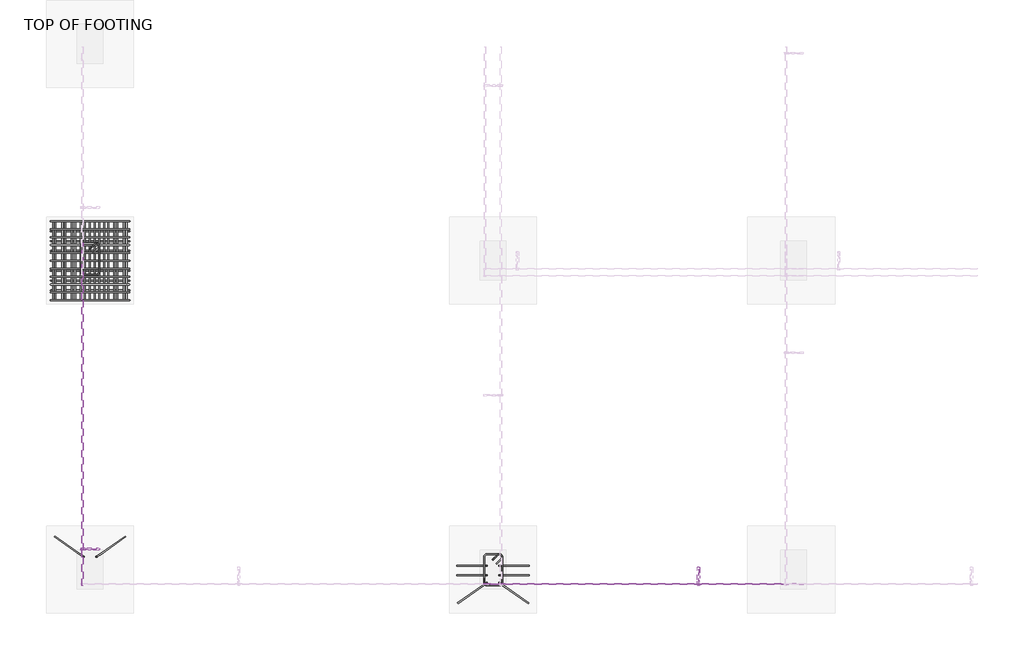
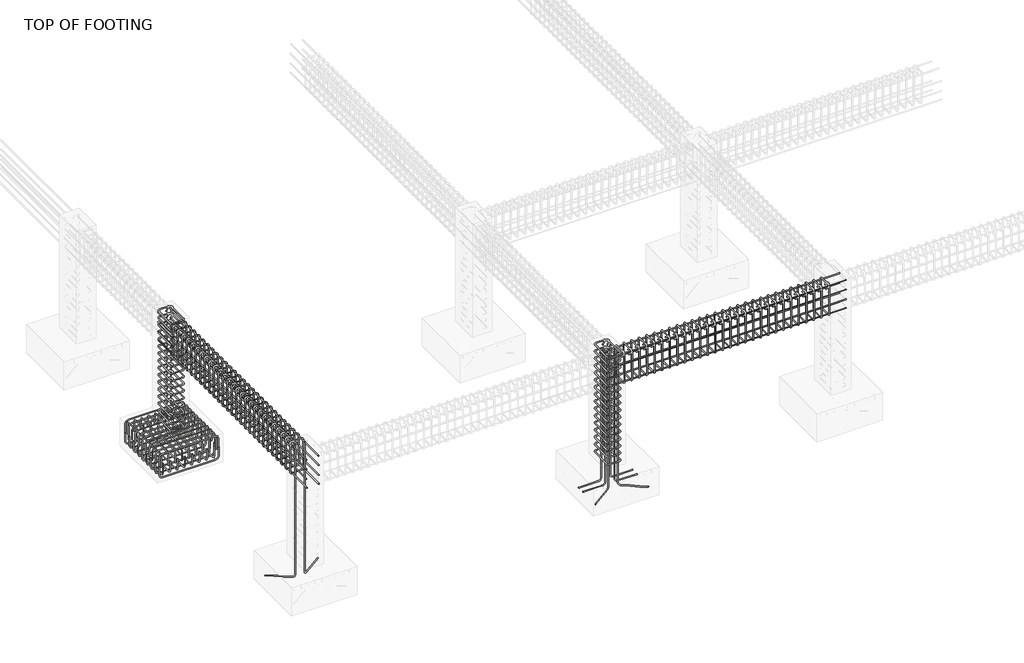
# One storey, part 3 of 13: 22 reinforcing bars.
"""IFC4 building model written with IfcOpenShell, lengths in millimetres."""

from ifc_helpers import new_model, si_unit, point, frame, origin, place, context, project, spatial, polyline, circle_curve, trimmed, segment, composite_curve, source, transform, mapped, element, save
from ifc_brep_helpers import swept_disk

model = new_model("IFC4")

# Units and contexts
model_context = context("Model", 3, world=origin())
ifc_project = project(units=[si_unit("LENGTHUNIT", "METRE", prefix="MILLI")], contexts=[model_context])

# Site, building, storey
site = spatial("IfcSite", under=ifc_project)
building = spatial("IfcBuilding", under=site)
storey = spatial("IfcBuildingStorey", under=building, Name="TOP OF FOOTING", Elevation=-1828.8)

# Reinforcing bars
placement = place(None, origin())
reinforcing_bar_shape = source(origin(), model_context, "Body", "SolidModel", [
    swept_disk(composite_curve([segment(polyline([(-6869.8542006, -257.8398401, -2046.7304597), (-6869.8542006, -257.8398401, -2194.0304597)]), True, "CONTINUOUS"), segment(trimmed(circle_curve(frame((-6916.2042006, -257.8398401, -2194.0304597), z_axis=(0.0, 1.0, 0.0), x_axis=(46.350000000000364, 0.0, 0.0)), 46.35), [point((-6869.8542006, -257.8398401, -2194.0304597))], [point((-6916.2042006, -257.8398401, -2240.3804597))], True, "CARTESIAN"), True, "CONTINUOUS"), segment(polyline([(-6916.2042006, -257.8398401, -2240.3804597), (-7730.8042006, -257.8398401, -2240.3804597)]), True, "CONTINUOUS"), segment(trimmed(circle_curve(frame((-7730.8042006, -257.8398401, -2194.0304597), z_axis=(0.0, 1.0, 0.0), x_axis=(0.0, 0.0, -46.34999999999991)), 46.35), [point((-7730.8042006, -257.8398401, -2240.3804597))], [point((-7777.1542006, -257.8398401, -2194.0304597))], True, "CARTESIAN"), True, "CONTINUOUS"), segment(polyline([(-7777.1542006, -257.8398401, -2194.0304597), (-7777.1542006, -257.8398401, -2046.7304597)]), True, "CONTINUOUS")], self_intersect=False), 6.35),
])
element("IfcReinforcingBar", 1, at=placement, inside=storey, context=model_context, shape_type="MappedRepresentation", body=[
    mapped(reinforcing_bar_shape, transform((0.0, 0.0, 0.0), x_axis=(1.0, 0.0, 0.0), y_axis=(0.0, 1.0, 0.0), z_axis=(0.0, 0.0, 1.0))),
    mapped(reinforcing_bar_shape, transform((0.0, -113.4125, 0.0), x_axis=(1.0, 0.0, 0.0), y_axis=(0.0, 1.0, 0.0), z_axis=(0.0, 0.0, 1.0))),
    mapped(reinforcing_bar_shape, transform((0.0, -226.825, 0.0), x_axis=(1.0, 0.0, 0.0), y_axis=(0.0, 1.0, 0.0), z_axis=(0.0, 0.0, 1.0))),
    mapped(reinforcing_bar_shape, transform((0.0, -340.2375, 0.0), x_axis=(1.0, 0.0, 0.0), y_axis=(0.0, 1.0, 0.0), z_axis=(0.0, 0.0, 1.0))),
    mapped(reinforcing_bar_shape, transform((0.0, -453.65, 0.0), x_axis=(1.0, 0.0, 0.0), y_axis=(0.0, 1.0, 0.0), z_axis=(0.0, 0.0, 1.0))),
    mapped(reinforcing_bar_shape, transform((0.0, -567.0625, 0.0), x_axis=(1.0, 0.0, 0.0), y_axis=(0.0, 1.0, 0.0), z_axis=(0.0, 0.0, 1.0))),
    mapped(reinforcing_bar_shape, transform((0.0, -680.475, 0.0), x_axis=(1.0, 0.0, 0.0), y_axis=(0.0, 1.0, 0.0), z_axis=(0.0, 0.0, 1.0))),
    mapped(reinforcing_bar_shape, transform((0.0, -793.8875, 0.0), x_axis=(1.0, 0.0, 0.0), y_axis=(0.0, 1.0, 0.0), z_axis=(0.0, 0.0, 1.0))),
    mapped(reinforcing_bar_shape, transform((0.0, -907.3, 0.0), x_axis=(1.0, 0.0, 0.0), y_axis=(0.0, 1.0, 0.0), z_axis=(0.0, 0.0, 1.0))),
])
reinforcing_bar_2_shape = source(origin(), model_context, "Body", "SolidModel", [
    swept_disk(composite_curve([segment(polyline([(-7777.3413042, -257.8398401, -2054.7114114), (-7777.3413042, -257.8398401, -1907.4114114)]), True, "CONTINUOUS"), segment(trimmed(circle_curve(frame((-7730.9913042, -257.8398401, -1907.4114114), z_axis=(0.0, 1.0, 0.0), x_axis=(-46.350000000000364, 0.0, 0.0)), 46.35), [point((-7777.3413042, -257.8398401, -1907.4114114))], [point((-7730.9913042, -257.8398401, -1861.0614114))], True, "CARTESIAN"), True, "CONTINUOUS"), segment(polyline([(-7730.9913042, -257.8398401, -1861.0614114), (-6918.3621718, -257.8398401, -1861.0614114)]), True, "CONTINUOUS"), segment(trimmed(circle_curve(frame((-6918.3621718, -257.8398401, -1907.4114114), z_axis=(0.0, 1.0, 0.0), x_axis=(0.0, 0.0, 46.34999999999991)), 46.35), [point((-6918.3621718, -257.8398401, -1861.0614114))], [point((-6872.0121718, -257.8398401, -1907.4114114))], True, "CARTESIAN"), True, "CONTINUOUS"), segment(polyline([(-6872.0121718, -257.8398401, -1907.4114114), (-6872.0121718, -257.8398401, -2054.7114114)]), True, "CONTINUOUS")], self_intersect=False), 6.35),
])
element("IfcReinforcingBar", 2, at=placement, inside=storey, context=model_context, shape_type="MappedRepresentation", body=[
    mapped(reinforcing_bar_2_shape, transform((0.0, 0.0, 0.0), x_axis=(1.0, 0.0, 0.0), y_axis=(0.0, 1.0, 0.0), z_axis=(0.0, 0.0, 1.0))),
    mapped(reinforcing_bar_2_shape, transform((0.0, -90.73, 0.0), x_axis=(1.0, 0.0, 0.0), y_axis=(0.0, 1.0, 0.0), z_axis=(0.0, 0.0, 1.0))),
    mapped(reinforcing_bar_2_shape, transform((0.0, -181.46, 0.0), x_axis=(1.0, 0.0, 0.0), y_axis=(0.0, 1.0, 0.0), z_axis=(0.0, 0.0, 1.0))),
    mapped(reinforcing_bar_2_shape, transform((0.0, -272.19, 0.0), x_axis=(1.0, 0.0, 0.0), y_axis=(0.0, 1.0, 0.0), z_axis=(0.0, 0.0, 1.0))),
    mapped(reinforcing_bar_2_shape, transform((0.0, -362.92, 0.0), x_axis=(1.0, 0.0, 0.0), y_axis=(0.0, 1.0, 0.0), z_axis=(0.0, 0.0, 1.0))),
    mapped(reinforcing_bar_2_shape, transform((0.0, -453.65, 0.0), x_axis=(1.0, 0.0, 0.0), y_axis=(0.0, 1.0, 0.0), z_axis=(0.0, 0.0, 1.0))),
    mapped(reinforcing_bar_2_shape, transform((0.0, -544.38, 0.0), x_axis=(1.0, 0.0, 0.0), y_axis=(0.0, 1.0, 0.0), z_axis=(0.0, 0.0, 1.0))),
    mapped(reinforcing_bar_2_shape, transform((0.0, -635.11, 0.0), x_axis=(1.0, 0.0, 0.0), y_axis=(0.0, 1.0, 0.0), z_axis=(0.0, 0.0, 1.0))),
    mapped(reinforcing_bar_2_shape, transform((0.0, -725.84, 0.0), x_axis=(1.0, 0.0, 0.0), y_axis=(0.0, 1.0, 0.0), z_axis=(0.0, 0.0, 1.0))),
    mapped(reinforcing_bar_2_shape, transform((0.0, -816.57, 0.0), x_axis=(1.0, 0.0, 0.0), y_axis=(0.0, 1.0, 0.0), z_axis=(0.0, 0.0, 1.0))),
    mapped(reinforcing_bar_2_shape, transform((0.0, -907.3, 0.0), x_axis=(1.0, 0.0, 0.0), y_axis=(0.0, 1.0, 0.0), z_axis=(0.0, 0.0, 1.0))),
])
reinforcing_bar_3_shape = source(origin(), model_context, "Body", "SolidModel", [
    swept_disk(composite_curve([segment(polyline([(-7721.4502846, -257.8398401, -2022.6645135), (-7721.4502846, -257.8398401, -2169.9645135)]), True, "CONTINUOUS"), segment(trimmed(circle_curve(frame((-7721.4502846, -304.1898401, -2169.9645135), z_axis=(-1.0, 0.0, 0.0), x_axis=(0.0, 46.35000000000002, 0.0)), 46.35), [point((-7721.4502846, -257.8398401, -2169.9645135))], [point((-7721.4502846, -304.1898401, -2216.3145135))], True, "CARTESIAN"), True, "CONTINUOUS"), segment(polyline([(-7721.4502846, -304.1898401, -2216.3145135), (-7721.4502846, -1118.7898401, -2216.3145135)]), True, "CONTINUOUS"), segment(trimmed(circle_curve(frame((-7721.4502846, -1118.7898401, -2169.9645135), z_axis=(-1.0, 0.0, 0.0), x_axis=(0.0, 0.0, -46.34999999999991)), 46.35), [point((-7721.4502846, -1118.7898401, -2216.3145135))], [point((-7721.4502846, -1165.1398401, -2169.9645135))], True, "CARTESIAN"), True, "CONTINUOUS"), segment(polyline([(-7721.4502846, -1165.1398401, -2169.9645135), (-7721.4502846, -1165.1398401, -2022.6645135)]), True, "CONTINUOUS")], self_intersect=False), 6.35),
])
element("IfcReinforcingBar", 3, at=placement, inside=storey, context=model_context, shape_type="MappedRepresentation", body=[
    mapped(reinforcing_bar_3_shape, transform((0.0, 0.0, 0.0), x_axis=(1.0, 0.0, 0.0), y_axis=(0.0, 1.0, 0.0), z_axis=(0.0, 0.0, 1.0))),
    mapped(reinforcing_bar_3_shape, transform((112.5551949, 0.0, 0.0), x_axis=(1.0, 0.0, 0.0), y_axis=(0.0, 1.0, 0.0), z_axis=(0.0, 0.0, 1.0))),
    mapped(reinforcing_bar_3_shape, transform((225.1103897, 0.0, 0.0), x_axis=(1.0, 0.0, 0.0), y_axis=(0.0, 1.0, 0.0), z_axis=(0.0, 0.0, 1.0))),
    mapped(reinforcing_bar_3_shape, transform((337.6655846, 0.0, 0.0), x_axis=(1.0, 0.0, 0.0), y_axis=(0.0, 1.0, 0.0), z_axis=(0.0, 0.0, 1.0))),
    mapped(reinforcing_bar_3_shape, transform((450.2207794, 0.0, 0.0), x_axis=(1.0, 0.0, 0.0), y_axis=(0.0, 1.0, 0.0), z_axis=(0.0, 0.0, 1.0))),
    mapped(reinforcing_bar_3_shape, transform((562.7759743, 0.0, 0.0), x_axis=(1.0, 0.0, 0.0), y_axis=(0.0, 1.0, 0.0), z_axis=(0.0, 0.0, 1.0))),
    mapped(reinforcing_bar_3_shape, transform((675.3311691, 0.0, 0.0), x_axis=(1.0, 0.0, 0.0), y_axis=(0.0, 1.0, 0.0), z_axis=(0.0, 0.0, 1.0))),
    mapped(reinforcing_bar_3_shape, transform((787.886364, 0.0, 0.0), x_axis=(1.0, 0.0, 0.0), y_axis=(0.0, 1.0, 0.0), z_axis=(0.0, 0.0, 1.0))),
])
reinforcing_bar_4_shape = source(origin(), model_context, "Body", "SolidModel", [
    swept_disk(composite_curve([segment(polyline([(-6905.0104502, -257.8398401, -2073.3758937), (-6905.0104502, -257.8398401, -1926.0758937)]), True, "CONTINUOUS"), segment(trimmed(circle_curve(frame((-6905.0104502, -304.1898401, -1926.0758937), z_axis=(1.0, 0.0, 0.0), x_axis=(0.0, 46.35000000000002, 0.0)), 46.35), [point((-6905.0104502, -257.8398401, -1926.0758937))], [point((-6905.0104502, -304.1898401, -1879.7258937))], True, "CARTESIAN"), True, "CONTINUOUS"), segment(polyline([(-6905.0104502, -304.1898401, -1879.7258937), (-6905.0104502, -1118.7898401, -1879.7258937)]), True, "CONTINUOUS"), segment(trimmed(circle_curve(frame((-6905.0104502, -1118.7898401, -1926.0758937), z_axis=(1.0, 0.0, 0.0), x_axis=(0.0, 0.0, 46.350000000000136)), 46.35), [point((-6905.0104502, -1118.7898401, -1879.7258937))], [point((-6905.0104502, -1165.1398401, -1926.0758937))], True, "CARTESIAN"), True, "CONTINUOUS"), segment(polyline([(-6905.0104502, -1165.1398401, -1926.0758937), (-6905.0104502, -1165.1398401, -2073.3758937)]), True, "CONTINUOUS")], self_intersect=False), 6.35),
])
element("IfcReinforcingBar", 4, at=placement, inside=storey, context=model_context, shape_type="MappedRepresentation", body=[
    mapped(reinforcing_bar_4_shape, transform((0.0, 0.0, 0.0), x_axis=(1.0, 0.0, 0.0), y_axis=(0.0, 1.0, 0.0), z_axis=(0.0, 0.0, 1.0))),
    mapped(reinforcing_bar_4_shape, transform((-105.0563863, 0.0, 0.0), x_axis=(1.0, 0.0, 0.0), y_axis=(0.0, 1.0, 0.0), z_axis=(0.0, 0.0, 1.0))),
    mapped(reinforcing_bar_4_shape, transform((-210.1127725, 0.0, 0.0), x_axis=(1.0, 0.0, 0.0), y_axis=(0.0, 1.0, 0.0), z_axis=(0.0, 0.0, 1.0))),
    mapped(reinforcing_bar_4_shape, transform((-315.1691588, 0.0, 0.0), x_axis=(1.0, 0.0, 0.0), y_axis=(0.0, 1.0, 0.0), z_axis=(0.0, 0.0, 1.0))),
    mapped(reinforcing_bar_4_shape, transform((-420.2255451, 0.0, 0.0), x_axis=(1.0, 0.0, 0.0), y_axis=(0.0, 1.0, 0.0), z_axis=(0.0, 0.0, 1.0))),
    mapped(reinforcing_bar_4_shape, transform((-525.2819314, 0.0, 0.0), x_axis=(1.0, 0.0, 0.0), y_axis=(0.0, 1.0, 0.0), z_axis=(0.0, 0.0, 1.0))),
    mapped(reinforcing_bar_4_shape, transform((-630.3383176, 0.0, 0.0), x_axis=(1.0, 0.0, 0.0), y_axis=(0.0, 1.0, 0.0), z_axis=(0.0, 0.0, 1.0))),
    mapped(reinforcing_bar_4_shape, transform((-735.3947039, 0.0, 0.0), x_axis=(1.0, 0.0, 0.0), y_axis=(0.0, 1.0, 0.0), z_axis=(0.0, 0.0, 1.0))),
    mapped(reinforcing_bar_4_shape, transform((-840.4510902, 0.0, 0.0), x_axis=(1.0, 0.0, 0.0), y_axis=(0.0, 1.0, 0.0), z_axis=(0.0, 0.0, 1.0))),
])
reinforcing_bar_5_shape = source(origin(), model_context, "Body", "SolidModel", [
    swept_disk(composite_curve([segment(polyline([(-7329.1155612, -577.7656055, -46.35), (-7273.3719982, -522.0220425, -46.35)]), True, "CONTINUOUS"), segment(trimmed(circle_curve(frame((-7251.2042006, -544.1898401, -46.35), z_axis=(0.0, 0.0, -1.0), x_axis=(-22.167797600000085, 22.16779759999997, 0.0)), 31.35), [point((-7273.3719982, -522.0220425, -46.35))], [point((-7219.8542006, -544.1898401, -46.35))], True, "CARTESIAN"), True, "CONTINUOUS"), segment(polyline([(-7219.8542006, -544.1898401, -46.35), (-7219.8542006, -838.7898401, -46.35)]), True, "CONTINUOUS"), segment(trimmed(circle_curve(frame((-7251.2042006, -838.7898401, -46.35), z_axis=(0.0, 0.0, -1.0), x_axis=(31.350000000000364, 0.0, 0.0)), 31.35), [point((-7219.8542006, -838.7898401, -46.35))], [point((-7251.2042006, -870.1398401, -46.35))], True, "CARTESIAN"), True, "CONTINUOUS"), segment(polyline([(-7251.2042006, -870.1398401, -46.35), (-7395.8042006, -870.1398401, -46.35)]), True, "CONTINUOUS"), segment(trimmed(circle_curve(frame((-7395.8042006, -838.8096252, -45.2363875), z_axis=(0.0, 0.035521928334481916, -0.9993688971583016), x_axis=(0.0, -31.330214899999987, -1.1136125000000021)), 31.35), [point((-7395.8042006, -870.1398401, -46.35))], [point((-7427.1542006, -838.8096252, -45.2363875))], True, "CARTESIAN"), True, "CONTINUOUS"), segment(polyline([(-7427.1542006, -838.8096252, -45.2363875), (-7427.1542006, -544.170055, -34.7636125)]), True, "CONTINUOUS"), segment(trimmed(circle_curve(frame((-7395.8042006, -544.170055, -34.7636125), z_axis=(0.0, 0.035521928334481916, -0.9993688971583016), x_axis=(-31.350000000000364, 0.0, 0.0)), 31.35), [point((-7427.1542006, -544.170055, -34.7636125))], [point((-7395.8042006, -512.8398401, -33.65))], True, "CARTESIAN"), True, "CONTINUOUS"), segment(polyline([(-7395.8042006, -512.8398401, -33.65), (-7251.2042006, -512.8398401, -33.65)]), True, "CONTINUOUS"), segment(trimmed(circle_curve(frame((-7251.2042006, -544.1898401, -33.65), z_axis=(0.0, 0.0, -1.0), x_axis=(0.0, 31.350000000000023, 0.0)), 31.35), [point((-7251.2042006, -512.8398401, -33.65))], [point((-7229.036403, -566.3576377, -33.65))], True, "CARTESIAN"), True, "CONTINUOUS"), segment(polyline([(-7229.036403, -566.3576377, -33.65), (-7284.779966, -622.1012007, -33.65)]), True, "CONTINUOUS")], self_intersect=False), 6.35),
])
element("IfcReinforcingBar", 5, at=placement, inside=storey, context=model_context, shape_type="MappedRepresentation", body=[
    mapped(reinforcing_bar_5_shape, transform((0.0, 0.0, 0.0), x_axis=(1.0, 0.0, 0.0), y_axis=(0.0, 1.0, 0.0), z_axis=(0.0, 0.0, 1.0))),
    mapped(reinforcing_bar_5_shape, transform((0.0, 0.0, -115.74), x_axis=(1.0, 0.0, 0.0), y_axis=(0.0, 1.0, 0.0), z_axis=(0.0, 0.0, 1.0))),
    mapped(reinforcing_bar_5_shape, transform((0.0, 0.0, -231.48), x_axis=(1.0, 0.0, 0.0), y_axis=(0.0, 1.0, 0.0), z_axis=(0.0, 0.0, 1.0))),
    mapped(reinforcing_bar_5_shape, transform((0.0, 0.0, -347.22), x_axis=(1.0, 0.0, 0.0), y_axis=(0.0, 1.0, 0.0), z_axis=(0.0, 0.0, 1.0))),
    mapped(reinforcing_bar_5_shape, transform((0.0, 0.0, -462.96), x_axis=(1.0, 0.0, 0.0), y_axis=(0.0, 1.0, 0.0), z_axis=(0.0, 0.0, 1.0))),
    mapped(reinforcing_bar_5_shape, transform((0.0, 0.0, -578.7), x_axis=(1.0, 0.0, 0.0), y_axis=(0.0, 1.0, 0.0), z_axis=(0.0, 0.0, 1.0))),
    mapped(reinforcing_bar_5_shape, transform((0.0, 0.0, -694.44), x_axis=(1.0, 0.0, 0.0), y_axis=(0.0, 1.0, 0.0), z_axis=(0.0, 0.0, 1.0))),
    mapped(reinforcing_bar_5_shape, transform((0.0, 0.0, -810.18), x_axis=(1.0, 0.0, 0.0), y_axis=(0.0, 1.0, 0.0), z_axis=(0.0, 0.0, 1.0))),
    mapped(reinforcing_bar_5_shape, transform((0.0, 0.0, -925.92), x_axis=(1.0, 0.0, 0.0), y_axis=(0.0, 1.0, 0.0), z_axis=(0.0, 0.0, 1.0))),
    mapped(reinforcing_bar_5_shape, transform((0.0, 0.0, -1041.66), x_axis=(1.0, 0.0, 0.0), y_axis=(0.0, 1.0, 0.0), z_axis=(0.0, 0.0, 1.0))),
    mapped(reinforcing_bar_5_shape, transform((0.0, 0.0, -1157.4), x_axis=(1.0, 0.0, 0.0), y_axis=(0.0, 1.0, 0.0), z_axis=(0.0, 0.0, 1.0))),
    mapped(reinforcing_bar_5_shape, transform((0.0, 0.0, -1273.14), x_axis=(1.0, 0.0, 0.0), y_axis=(0.0, 1.0, 0.0), z_axis=(0.0, 0.0, 1.0))),
    mapped(reinforcing_bar_5_shape, transform((0.0, 0.0, -1388.88), x_axis=(1.0, 0.0, 0.0), y_axis=(0.0, 1.0, 0.0), z_axis=(0.0, 0.0, 1.0))),
    mapped(reinforcing_bar_5_shape, transform((0.0, 0.0, -1504.62), x_axis=(1.0, 0.0, 0.0), y_axis=(0.0, 1.0, 0.0), z_axis=(0.0, 0.0, 1.0))),
    mapped(reinforcing_bar_5_shape, transform((0.0, 0.0, -1620.36), x_axis=(1.0, 0.0, 0.0), y_axis=(0.0, 1.0, 0.0), z_axis=(0.0, 0.0, 1.0))),
    mapped(reinforcing_bar_5_shape, transform((0.0, 0.0, -1736.1), x_axis=(1.0, 0.0, 0.0), y_axis=(0.0, 1.0, 0.0), z_axis=(0.0, 0.0, 1.0))),
])
element("IfcReinforcingBar", 6, at=placement, inside=storey, context=model_context, shape_type="SolidModel", body=[
    swept_disk(composite_curve([segment(polyline([(-7251.2042006, -4110.8336602, -40.0), (-7251.2042006, -4110.8336602, -2142.45)]), True, "CONTINUOUS"), segment(trimmed(circle_curve(frame((-7213.2365034, -4084.2483924, -2142.45), z_axis=(0.5735764363510318, -0.8191520442890019, 0.0), x_axis=(-37.96769719999975, -26.58526780000011, 0.0)), 46.35), [point((-7251.2042006, -4110.8336602, -2142.45))], [point((-7213.2365034, -4084.2483924, -2188.8))], True, "CARTESIAN"), True, "CONTINUOUS"), segment(polyline([(-7213.2365034, -4084.2483924, -2188.8), (-6917.2359122, -3876.9865471, -2188.8)]), True, "CONTINUOUS")], self_intersect=False), 6.35),
])
element("IfcReinforcingBar", 7, at=placement, inside=storey, context=model_context, shape_type="SolidModel", body=[
    swept_disk(composite_curve([segment(polyline([(-7395.8042006, -4110.8336602, -40.0), (-7395.8042006, -4110.8336602, -2142.45)]), True, "CONTINUOUS"), segment(trimmed(circle_curve(frame((-7433.7718979, -4084.2483924, -2142.45), z_axis=(0.5735764363510226, 0.8191520442890082, 0.0), x_axis=(37.96769730000051, -26.58526780000011, 0.0)), 46.35), [point((-7395.8042006, -4110.8336602, -2142.45))], [point((-7433.7718979, -4084.2483924, -2188.8))], True, "CARTESIAN"), True, "CONTINUOUS"), segment(polyline([(-7433.7718979, -4084.2483924, -2188.8), (-7729.7724891, -3876.9865471, -2188.8)]), True, "CONTINUOUS")], self_intersect=False), 6.35),
])
reinforcing_bar_6_shape = source(origin(), model_context, "Body", "SolidModel", [
    swept_disk(composite_curve([segment(polyline([(-2701.3703668, -4145.7099889, -46.35), (-2645.6268039, -4089.966426, -46.35)]), True, "CONTINUOUS"), segment(trimmed(circle_curve(frame((-2623.4590063, -4112.1342236, -46.35), z_axis=(0.0, 0.0, -1.0), x_axis=(-22.167797600000085, 22.167797600000085, 0.0)), 31.35), [point((-2645.6268039, -4089.966426, -46.35))], [point((-2592.1090063, -4112.1342236, -46.35))], True, "CARTESIAN"), True, "CONTINUOUS"), segment(polyline([(-2592.1090063, -4112.1342236, -46.35), (-2592.1090063, -4406.7342236, -46.35)]), True, "CONTINUOUS"), segment(trimmed(circle_curve(frame((-2623.4590063, -4406.7342236, -46.35), z_axis=(0.0, 0.0, -1.0), x_axis=(31.34999999999991, 0.0, 0.0)), 31.35), [point((-2592.1090063, -4406.7342236, -46.35))], [point((-2623.4590063, -4438.0842236, -46.35))], True, "CARTESIAN"), True, "CONTINUOUS"), segment(polyline([(-2623.4590063, -4438.0842236, -46.35), (-2768.0590063, -4438.0842236, -46.35)]), True, "CONTINUOUS"), segment(trimmed(circle_curve(frame((-2768.0590063, -4406.7540087, -45.2363875), z_axis=(0.0, 0.035521928334481916, -0.9993688971583016), x_axis=(0.0, -31.3302149000001, -1.1136125000000021)), 31.35), [point((-2768.0590063, -4438.0842236, -46.35))], [point((-2799.4090063, -4406.7540087, -45.2363875))], True, "CARTESIAN"), True, "CONTINUOUS"), segment(polyline([(-2799.4090063, -4406.7540087, -45.2363875), (-2799.4090063, -4112.1144385, -34.7636125)]), True, "CONTINUOUS"), segment(trimmed(circle_curve(frame((-2768.0590063, -4112.1144385, -34.7636125), z_axis=(0.0, 0.035521928334481916, -0.9993688971583016), x_axis=(-31.34999999999991, 0.0, 0.0)), 31.35), [point((-2799.4090063, -4112.1144385, -34.7636125))], [point((-2768.0590063, -4080.7842236, -33.65))], True, "CARTESIAN"), True, "CONTINUOUS"), segment(polyline([(-2768.0590063, -4080.7842236, -33.65), (-2623.4590063, -4080.7842236, -33.65)]), True, "CONTINUOUS"), segment(trimmed(circle_curve(frame((-2623.4590063, -4112.1342236, -33.65), z_axis=(0.0, 0.0, -1.0), x_axis=(0.0, 31.34999999999991, 0.0)), 31.35), [point((-2623.4590063, -4080.7842236, -33.65))], [point((-2601.2912087, -4134.3020212, -33.65))], True, "CARTESIAN"), True, "CONTINUOUS"), segment(polyline([(-2601.2912087, -4134.3020212, -33.65), (-2657.0347716, -4190.0455841, -33.65)]), True, "CONTINUOUS")], self_intersect=False), 6.35),
])
element("IfcReinforcingBar", 8, at=placement, inside=storey, context=model_context, shape_type="MappedRepresentation", body=[
    mapped(reinforcing_bar_6_shape, transform((0.0, 0.0, 0.0), x_axis=(1.0, 0.0, 0.0), y_axis=(0.0, 1.0, 0.0), z_axis=(0.0, 0.0, 1.0))),
    mapped(reinforcing_bar_6_shape, transform((0.0, 0.0, -115.74), x_axis=(1.0, 0.0, 0.0), y_axis=(0.0, 1.0, 0.0), z_axis=(0.0, 0.0, 1.0))),
    mapped(reinforcing_bar_6_shape, transform((0.0, 0.0, -231.48), x_axis=(1.0, 0.0, 0.0), y_axis=(0.0, 1.0, 0.0), z_axis=(0.0, 0.0, 1.0))),
    mapped(reinforcing_bar_6_shape, transform((0.0, 0.0, -347.22), x_axis=(1.0, 0.0, 0.0), y_axis=(0.0, 1.0, 0.0), z_axis=(0.0, 0.0, 1.0))),
    mapped(reinforcing_bar_6_shape, transform((0.0, 0.0, -462.96), x_axis=(1.0, 0.0, 0.0), y_axis=(0.0, 1.0, 0.0), z_axis=(0.0, 0.0, 1.0))),
    mapped(reinforcing_bar_6_shape, transform((0.0, 0.0, -578.7), x_axis=(1.0, 0.0, 0.0), y_axis=(0.0, 1.0, 0.0), z_axis=(0.0, 0.0, 1.0))),
    mapped(reinforcing_bar_6_shape, transform((0.0, 0.0, -694.44), x_axis=(1.0, 0.0, 0.0), y_axis=(0.0, 1.0, 0.0), z_axis=(0.0, 0.0, 1.0))),
    mapped(reinforcing_bar_6_shape, transform((0.0, 0.0, -810.18), x_axis=(1.0, 0.0, 0.0), y_axis=(0.0, 1.0, 0.0), z_axis=(0.0, 0.0, 1.0))),
    mapped(reinforcing_bar_6_shape, transform((0.0, 0.0, -925.92), x_axis=(1.0, 0.0, 0.0), y_axis=(0.0, 1.0, 0.0), z_axis=(0.0, 0.0, 1.0))),
    mapped(reinforcing_bar_6_shape, transform((0.0, 0.0, -1041.66), x_axis=(1.0, 0.0, 0.0), y_axis=(0.0, 1.0, 0.0), z_axis=(0.0, 0.0, 1.0))),
    mapped(reinforcing_bar_6_shape, transform((0.0, 0.0, -1157.4), x_axis=(1.0, 0.0, 0.0), y_axis=(0.0, 1.0, 0.0), z_axis=(0.0, 0.0, 1.0))),
    mapped(reinforcing_bar_6_shape, transform((0.0, 0.0, -1273.14), x_axis=(1.0, 0.0, 0.0), y_axis=(0.0, 1.0, 0.0), z_axis=(0.0, 0.0, 1.0))),
    mapped(reinforcing_bar_6_shape, transform((0.0, 0.0, -1388.88), x_axis=(1.0, 0.0, 0.0), y_axis=(0.0, 1.0, 0.0), z_axis=(0.0, 0.0, 1.0))),
    mapped(reinforcing_bar_6_shape, transform((0.0, 0.0, -1504.62), x_axis=(1.0, 0.0, 0.0), y_axis=(0.0, 1.0, 0.0), z_axis=(0.0, 0.0, 1.0))),
    mapped(reinforcing_bar_6_shape, transform((0.0, 0.0, -1620.36), x_axis=(1.0, 0.0, 0.0), y_axis=(0.0, 1.0, 0.0), z_axis=(0.0, 0.0, 1.0))),
    mapped(reinforcing_bar_6_shape, transform((0.0, 0.0, -1736.1), x_axis=(1.0, 0.0, 0.0), y_axis=(0.0, 1.0, 0.0), z_axis=(0.0, 0.0, 1.0))),
])
element("IfcReinforcingBar", 9, at=placement, inside=storey, context=model_context, shape_type="SolidModel", body=[
    swept_disk(composite_curve([segment(polyline([(-2623.4590063, -4408.0347869, -40.0), (-2623.4590063, -4408.0347869, -2142.45)]), True, "CONTINUOUS"), segment(trimmed(circle_curve(frame((-2585.491309, -4434.6200547, -2142.45), z_axis=(-0.5735764363510132, -0.8191520442890149, 0.0), x_axis=(-37.967697300000054, 26.58526780000011, 0.0)), 46.35), [point((-2623.4590063, -4408.0347869, -2142.45))], [point((-2585.491309, -4434.6200547, -2188.8))], True, "CARTESIAN"), True, "CONTINUOUS"), segment(polyline([(-2585.491309, -4434.6200547, -2188.8), (-2289.4907178, -4641.8819, -2188.8)]), True, "CONTINUOUS")], self_intersect=False), 6.35),
])
element("IfcReinforcingBar", 10, at=placement, inside=storey, context=model_context, shape_type="SolidModel", body=[
    swept_disk(composite_curve([segment(polyline([(-2768.0590063, -4408.0347869, -40.0), (-2768.0590063, -4408.0347869, -2142.45)]), True, "CONTINUOUS"), segment(trimmed(circle_curve(frame((-2806.0267035, -4434.6200547, -2142.45), z_axis=(-0.5735764363510413, 0.8191520442889952, 0.0), x_axis=(37.9676972000002, 26.58526780000011, 0.0)), 46.35), [point((-2768.0590063, -4408.0347869, -2142.45))], [point((-2806.0267035, -4434.6200547, -2188.8))], True, "CARTESIAN"), True, "CONTINUOUS"), segment(polyline([(-2806.0267035, -4434.6200547, -2188.8), (-3102.0272947, -4641.8819, -2188.8)]), True, "CONTINUOUS")], self_intersect=False), 6.35),
])
reinforcing_bar_7_shape = source(origin(), model_context, "Body", "SolidModel", [
    swept_disk(composite_curve([segment(polyline([(-2768.0590063, -4212.4451378, -40.0), (-2768.0590063, -4212.4451378, -2135.3077585)]), True, "CONTINUOUS"), segment(trimmed(circle_curve(frame((-2814.4090063, -4212.4451378, -2135.3077585), z_axis=(0.0, 1.0, 0.0), x_axis=(46.34999999999991, 0.0, 0.0)), 46.35), [point((-2768.0590063, -4212.4451378, -2135.3077585))], [point((-2814.4090063, -4212.4451378, -2181.6577585))], True, "CARTESIAN"), True, "CONTINUOUS"), segment(polyline([(-2814.4090063, -4212.4451378, -2181.6577585), (-3110.7307379, -4212.4451378, -2181.6577585)]), True, "CONTINUOUS")], self_intersect=False), 6.35),
])
element("IfcReinforcingBar", 11, at=placement, inside=storey, context=model_context, shape_type="MappedRepresentation", body=[
    mapped(reinforcing_bar_7_shape, transform((0.0, 0.0, 0.0), x_axis=(1.0, 0.0, 0.0), y_axis=(0.0, 1.0, 0.0), z_axis=(0.0, 0.0, 1.0))),
    mapped(reinforcing_bar_7_shape, transform((0.0, -110.4020916, 0.0), x_axis=(1.0, 0.0, 0.0), y_axis=(0.0, 1.0, 0.0), z_axis=(0.0, 0.0, 1.0))),
])
reinforcing_bar_8_shape = source(origin(), model_context, "Body", "SolidModel", [
    swept_disk(composite_curve([segment(polyline([(-2625.804081, -4212.4451378, -40.0), (-2625.804081, -4212.4451378, -2135.3077585)]), True, "CONTINUOUS"), segment(trimmed(circle_curve(frame((-2579.454081, -4212.4451378, -2135.3077585), z_axis=(0.0, -1.0, 0.0), x_axis=(-46.350000000000364, 0.0, 0.0)), 46.35), [point((-2625.804081, -4212.4451378, -2135.3077585))], [point((-2579.454081, -4212.4451378, -2181.6577585))], True, "CARTESIAN"), True, "CONTINUOUS"), segment(polyline([(-2579.454081, -4212.4451378, -2181.6577585), (-2283.1323494, -4212.4451378, -2181.6577585)]), True, "CONTINUOUS")], self_intersect=False), 6.35),
])
element("IfcReinforcingBar", 12, at=placement, inside=storey, context=model_context, shape_type="MappedRepresentation", body=[
    mapped(reinforcing_bar_8_shape, transform((0.0, 0.0, 0.0), x_axis=(1.0, 0.0, 0.0), y_axis=(0.0, 1.0, 0.0), z_axis=(0.0, 0.0, 1.0))),
    mapped(reinforcing_bar_8_shape, transform((0.0, -110.4020916, 0.0), x_axis=(1.0, 0.0, 0.0), y_axis=(0.0, 1.0, 0.0), z_axis=(0.0, 0.0, 1.0))),
])
reinforcing_bar_9_shape = source(origin(), model_context, "Body", "SolidModel", [
    swept_disk(composite_curve([segment(polyline([(-7317.8928401, -922.8398401, -111.2757654), (-7373.636403, -922.8398401, -55.5322024)]), True, "CONTINUOUS"), segment(trimmed(circle_curve(frame((-7395.8042006, -922.8398401, -77.7), z_axis=(0.0, -1.0, 0.0), x_axis=(22.167797599999176, 0.0, 22.1677976)), 31.35), [point((-7373.636403, -922.8398401, -55.5322024))], [point((-7427.1542006, -922.8398401, -77.7))], True, "CARTESIAN"), True, "CONTINUOUS"), segment(polyline([(-7427.1542006, -922.8398401, -77.7), (-7427.1542006, -922.8398401, -522.3)]), True, "CONTINUOUS"), segment(trimmed(circle_curve(frame((-7395.8042006, -922.8398401, -522.3), z_axis=(0.0, -1.0, 0.0), x_axis=(-31.350000000000364, 0.0, 0.0)), 31.35), [point((-7427.1542006, -922.8398401, -522.3))], [point((-7395.8042006, -922.8398401, -553.65))], True, "CARTESIAN"), True, "CONTINUOUS"), segment(polyline([(-7395.8042006, -922.8398401, -553.65), (-7251.2042006, -922.8398401, -553.65)]), True, "CONTINUOUS"), segment(trimmed(circle_curve(frame((-7251.2042006, -922.0552545, -522.3098193), z_axis=(0.0, -0.9996867842138424, 0.02502665515378633), x_axis=(0.0, -0.7845855999999003, -31.34018070000002)), 31.35), [point((-7251.2042006, -922.8398401, -553.65))], [point((-7219.8542006, -922.0552545, -522.3098193))], True, "CARTESIAN"), True, "CONTINUOUS"), segment(polyline([(-7219.8542006, -922.0552545, -522.3098193), (-7219.8542006, -910.9244258, -77.6901807)]), True, "CONTINUOUS"), segment(trimmed(circle_curve(frame((-7251.2042006, -910.9244258, -77.6901807), z_axis=(0.0, -0.9996867842138424, 0.02502665515378633), x_axis=(31.350000000000364, 0.0, 0.0)), 31.35), [point((-7219.8542006, -910.9244258, -77.6901807))], [point((-7251.2042006, -910.1398401, -46.35))], True, "CARTESIAN"), True, "CONTINUOUS"), segment(polyline([(-7251.2042006, -910.1398401, -46.35), (-7395.8042006, -910.1398401, -46.35)]), True, "CONTINUOUS"), segment(trimmed(circle_curve(frame((-7395.8042006, -910.1398401, -77.7), z_axis=(0.0, -1.0, 0.0), x_axis=(0.0, 0.0, 31.35)), 31.35), [point((-7395.8042006, -910.1398401, -46.35))], [point((-7417.9719982, -910.1398401, -99.8677976))], True, "CARTESIAN"), True, "CONTINUOUS"), segment(polyline([(-7417.9719982, -910.1398401, -99.8677976), (-7362.2284353, -910.1398401, -155.6113605)]), True, "CONTINUOUS")], self_intersect=False), 6.35),
])
element("IfcReinforcingBar", 13, at=placement, inside=storey, context=model_context, shape_type="MappedRepresentation", body=[
    mapped(reinforcing_bar_9_shape, transform((0.0, 0.0, 0.0), x_axis=(1.0, 0.0, 0.0), y_axis=(0.0, 1.0, 0.0), z_axis=(0.0, 0.0, 1.0))),
    mapped(reinforcing_bar_9_shape, transform((0.0, -119.4324763, 0.0), x_axis=(1.0, 0.0, 0.0), y_axis=(0.0, 1.0, 0.0), z_axis=(0.0, 0.0, 1.0))),
    mapped(reinforcing_bar_9_shape, transform((0.0, -238.8649526, 0.0), x_axis=(1.0, 0.0, 0.0), y_axis=(0.0, 1.0, 0.0), z_axis=(0.0, 0.0, 1.0))),
    mapped(reinforcing_bar_9_shape, transform((0.0, -358.2974289, 0.0), x_axis=(1.0, 0.0, 0.0), y_axis=(0.0, 1.0, 0.0), z_axis=(0.0, 0.0, 1.0))),
    mapped(reinforcing_bar_9_shape, transform((0.0, -477.7299051, 0.0), x_axis=(1.0, 0.0, 0.0), y_axis=(0.0, 1.0, 0.0), z_axis=(0.0, 0.0, 1.0))),
    mapped(reinforcing_bar_9_shape, transform((0.0, -597.1623814, 0.0), x_axis=(1.0, 0.0, 0.0), y_axis=(0.0, 1.0, 0.0), z_axis=(0.0, 0.0, 1.0))),
    mapped(reinforcing_bar_9_shape, transform((0.0, -716.5948577, 0.0), x_axis=(1.0, 0.0, 0.0), y_axis=(0.0, 1.0, 0.0), z_axis=(0.0, 0.0, 1.0))),
    mapped(reinforcing_bar_9_shape, transform((0.0, -836.027334, 0.0), x_axis=(1.0, 0.0, 0.0), y_axis=(0.0, 1.0, 0.0), z_axis=(0.0, 0.0, 1.0))),
    mapped(reinforcing_bar_9_shape, transform((0.0, -955.4598103, 0.0), x_axis=(1.0, 0.0, 0.0), y_axis=(0.0, 1.0, 0.0), z_axis=(0.0, 0.0, 1.0))),
    mapped(reinforcing_bar_9_shape, transform((0.0, -1074.8922866, 0.0), x_axis=(1.0, 0.0, 0.0), y_axis=(0.0, 1.0, 0.0), z_axis=(0.0, 0.0, 1.0))),
    mapped(reinforcing_bar_9_shape, transform((0.0, -1194.3247629, 0.0), x_axis=(1.0, 0.0, 0.0), y_axis=(0.0, 1.0, 0.0), z_axis=(0.0, 0.0, 1.0))),
    mapped(reinforcing_bar_9_shape, transform((0.0, -1313.7572392, 0.0), x_axis=(1.0, 0.0, 0.0), y_axis=(0.0, 1.0, 0.0), z_axis=(0.0, 0.0, 1.0))),
    mapped(reinforcing_bar_9_shape, transform((0.0, -1433.1897154, 0.0), x_axis=(1.0, 0.0, 0.0), y_axis=(0.0, 1.0, 0.0), z_axis=(0.0, 0.0, 1.0))),
    mapped(reinforcing_bar_9_shape, transform((0.0, -1552.6221917, 0.0), x_axis=(1.0, 0.0, 0.0), y_axis=(0.0, 1.0, 0.0), z_axis=(0.0, 0.0, 1.0))),
    mapped(reinforcing_bar_9_shape, transform((0.0, -1672.054668, 0.0), x_axis=(1.0, 0.0, 0.0), y_axis=(0.0, 1.0, 0.0), z_axis=(0.0, 0.0, 1.0))),
    mapped(reinforcing_bar_9_shape, transform((0.0, -1791.4871443, 0.0), x_axis=(1.0, 0.0, 0.0), y_axis=(0.0, 1.0, 0.0), z_axis=(0.0, 0.0, 1.0))),
    mapped(reinforcing_bar_9_shape, transform((0.0, -1910.9196206, 0.0), x_axis=(1.0, 0.0, 0.0), y_axis=(0.0, 1.0, 0.0), z_axis=(0.0, 0.0, 1.0))),
    mapped(reinforcing_bar_9_shape, transform((0.0, -2030.3520969, 0.0), x_axis=(1.0, 0.0, 0.0), y_axis=(0.0, 1.0, 0.0), z_axis=(0.0, 0.0, 1.0))),
    mapped(reinforcing_bar_9_shape, transform((0.0, -2149.7845732, 0.0), x_axis=(1.0, 0.0, 0.0), y_axis=(0.0, 1.0, 0.0), z_axis=(0.0, 0.0, 1.0))),
    mapped(reinforcing_bar_9_shape, transform((0.0, -2269.2170495, 0.0), x_axis=(1.0, 0.0, 0.0), y_axis=(0.0, 1.0, 0.0), z_axis=(0.0, 0.0, 1.0))),
    mapped(reinforcing_bar_9_shape, transform((0.0, -2388.6495257, 0.0), x_axis=(1.0, 0.0, 0.0), y_axis=(0.0, 1.0, 0.0), z_axis=(0.0, 0.0, 1.0))),
    mapped(reinforcing_bar_9_shape, transform((0.0, -2508.082002, 0.0), x_axis=(1.0, 0.0, 0.0), y_axis=(0.0, 1.0, 0.0), z_axis=(0.0, 0.0, 1.0))),
    mapped(reinforcing_bar_9_shape, transform((0.0, -2627.5144783, 0.0), x_axis=(1.0, 0.0, 0.0), y_axis=(0.0, 1.0, 0.0), z_axis=(0.0, 0.0, 1.0))),
    mapped(reinforcing_bar_9_shape, transform((0.0, -2746.9469546, 0.0), x_axis=(1.0, 0.0, 0.0), y_axis=(0.0, 1.0, 0.0), z_axis=(0.0, 0.0, 1.0))),
    mapped(reinforcing_bar_9_shape, transform((0.0, -2866.3794309, 0.0), x_axis=(1.0, 0.0, 0.0), y_axis=(0.0, 1.0, 0.0), z_axis=(0.0, 0.0, 1.0))),
    mapped(reinforcing_bar_9_shape, transform((0.0, -2985.8119072, 0.0), x_axis=(1.0, 0.0, 0.0), y_axis=(0.0, 1.0, 0.0), z_axis=(0.0, 0.0, 1.0))),
    mapped(reinforcing_bar_9_shape, transform((0.0, -3105.2443835, 0.0), x_axis=(1.0, 0.0, 0.0), y_axis=(0.0, 1.0, 0.0), z_axis=(0.0, 0.0, 1.0))),
])
reinforcing_bar_10_shape = source(origin(), model_context, "Body", "SolidModel", [
    swept_disk(composite_curve([segment(polyline([(-7232.5542006, -506.4898401, -77.7), (-7232.5542006, -4444.4342236, -77.7)]), True, "CONTINUOUS")], self_intersect=False), 6.35),
])
element("IfcReinforcingBar", 14, at=placement, inside=storey, context=model_context, shape_type="MappedRepresentation", body=[
    mapped(reinforcing_bar_10_shape, transform((0.0, 0.0, 0.0), x_axis=(1.0, 0.0, 0.0), y_axis=(0.0, 1.0, 0.0), z_axis=(0.0, 0.0, 1.0))),
    mapped(reinforcing_bar_10_shape, transform((-181.9, 0.0, 0.0), x_axis=(1.0, 0.0, 0.0), y_axis=(0.0, 1.0, 0.0), z_axis=(0.0, 0.0, 1.0))),
])
reinforcing_bar_11_shape = source(origin(), model_context, "Body", "SolidModel", [
    swept_disk(composite_curve([segment(polyline([(-7226.2853665, -506.4898401, -535.4875415), (-7226.2853665, -4444.4342236, -535.4875415)]), True, "CONTINUOUS")], self_intersect=False), 6.35),
])
element("IfcReinforcingBar", 15, at=placement, inside=storey, context=model_context, shape_type="MappedRepresentation", body=[
    mapped(reinforcing_bar_11_shape, transform((0.0, 0.0, 0.0), x_axis=(1.0, 0.0, 0.0), y_axis=(0.0, 1.0, 0.0), z_axis=(0.0, 0.0, 1.0))),
    mapped(reinforcing_bar_11_shape, transform((-182.7063756, 0.0, 0.0), x_axis=(1.0, 0.0, 0.0), y_axis=(0.0, 1.0, 0.0), z_axis=(0.0, 0.0, 1.0))),
])
reinforcing_bar_12_shape = source(origin(), model_context, "Body", "SolidModel", [
    swept_disk(composite_curve([segment(polyline([(-7226.2853665, -506.4898401, -392.3), (-7226.2853665, -4444.4342236, -392.3)]), True, "CONTINUOUS")], self_intersect=False), 6.35),
])
element("IfcReinforcingBar", 16, at=placement, inside=storey, context=model_context, shape_type="MappedRepresentation", body=[
    mapped(reinforcing_bar_12_shape, transform((0.0, 0.0, 0.0), x_axis=(1.0, 0.0, 0.0), y_axis=(0.0, 1.0, 0.0), z_axis=(0.0, 0.0, 1.0))),
    mapped(reinforcing_bar_12_shape, transform((-188.4461921, 0.0, 0.0), x_axis=(1.0, 0.0, 0.0), y_axis=(0.0, 1.0, 0.0), z_axis=(0.0, 0.0, 1.0))),
])
reinforcing_bar_13_shape = source(origin(), model_context, "Body", "SolidModel", [
    swept_disk(composite_curve([segment(polyline([(-7226.2853665, -506.4898401, -232.3), (-7226.2853665, -4444.4342236, -232.3)]), True, "CONTINUOUS")], self_intersect=False), 6.35),
])
element("IfcReinforcingBar", 17, at=placement, inside=storey, context=model_context, shape_type="MappedRepresentation", body=[
    mapped(reinforcing_bar_13_shape, transform((0.0, 0.0, 0.0), x_axis=(1.0, 0.0, 0.0), y_axis=(0.0, 1.0, 0.0), z_axis=(0.0, 0.0, 1.0))),
    mapped(reinforcing_bar_13_shape, transform((-188.4461921, 0.0, 0.0), x_axis=(1.0, 0.0, 0.0), y_axis=(0.0, 1.0, 0.0), z_axis=(0.0, 0.0, 1.0))),
])
reinforcing_bar_14_shape = source(origin(), model_context, "Body", "SolidModel", [
    swept_disk(composite_curve([segment(polyline([(-2539.4090063, -4328.822863, -111.2757654), (-2539.4090063, -4384.566426, -55.5322024)]), True, "CONTINUOUS"), segment(trimmed(circle_curve(frame((-2539.4090063, -4406.7342236, -77.7), z_axis=(1.0, 0.0, 0.0), x_axis=(0.0, 22.167797600000085, 22.1677976)), 31.35), [point((-2539.4090063, -4384.566426, -55.5322024))], [point((-2539.4090063, -4438.0842236, -77.7))], True, "CARTESIAN"), True, "CONTINUOUS"), segment(polyline([(-2539.4090063, -4438.0842236, -77.7), (-2539.4090063, -4438.0842236, -522.3)]), True, "CONTINUOUS"), segment(trimmed(circle_curve(frame((-2539.4090063, -4406.7342236, -522.3), z_axis=(1.0, 0.0, 0.0), x_axis=(0.0, -31.349999999999454, 0.0)), 31.35), [point((-2539.4090063, -4438.0842236, -522.3))], [point((-2539.4090063, -4406.7342236, -553.65))], True, "CARTESIAN"), True, "CONTINUOUS"), segment(polyline([(-2539.4090063, -4406.7342236, -553.65), (-2539.4090063, -4262.1342236, -553.65)]), True, "CONTINUOUS"), segment(trimmed(circle_curve(frame((-2540.1935919, -4262.1342236, -522.3098193), z_axis=(0.9996867842138424, 0.0, 0.02502665515378633), x_axis=(0.7845855999999003, 0.0, -31.34018070000002)), 31.35), [point((-2539.4090063, -4262.1342236, -553.65))], [point((-2540.1935919, -4230.7842236, -522.3098193))], True, "CARTESIAN"), True, "CONTINUOUS"), segment(polyline([(-2540.1935919, -4230.7842236, -522.3098193), (-2551.3244206, -4230.7842236, -77.6901807)]), True, "CONTINUOUS"), segment(trimmed(circle_curve(frame((-2551.3244206, -4262.1342236, -77.6901807), z_axis=(0.9996867842138424, 0.0, 0.02502665515378633), x_axis=(0.0, 31.350000000000364, 0.0)), 31.35), [point((-2551.3244206, -4230.7842236, -77.6901807))], [point((-2552.1090063, -4262.1342236, -46.35))], True, "CARTESIAN"), True, "CONTINUOUS"), segment(polyline([(-2552.1090063, -4262.1342236, -46.35), (-2552.1090063, -4406.7342236, -46.35)]), True, "CONTINUOUS"), segment(trimmed(circle_curve(frame((-2552.1090063, -4406.7342236, -77.7), z_axis=(1.0, 0.0, 0.0), x_axis=(0.0, 0.0, 31.35)), 31.35), [point((-2552.1090063, -4406.7342236, -46.35))], [point((-2552.1090063, -4428.9020212, -99.8677976))], True, "CARTESIAN"), True, "CONTINUOUS"), segment(polyline([(-2552.1090063, -4428.9020212, -99.8677976), (-2552.1090063, -4373.1584582, -155.6113605)]), True, "CONTINUOUS")], self_intersect=False), 6.35),
])
element("IfcReinforcingBar", 18, at=placement, inside=storey, context=model_context, shape_type="MappedRepresentation", body=[
    mapped(reinforcing_bar_14_shape, transform((0.0, 0.0, 0.0), x_axis=(1.0, 0.0, 0.0), y_axis=(0.0, 1.0, 0.0), z_axis=(0.0, 0.0, 1.0))),
    mapped(reinforcing_bar_14_shape, transform((116.2425191, 0.0, 0.0), x_axis=(1.0, 0.0, 0.0), y_axis=(0.0, 1.0, 0.0), z_axis=(0.0, 0.0, 1.0))),
    mapped(reinforcing_bar_14_shape, transform((232.4850382, 0.0, 0.0), x_axis=(1.0, 0.0, 0.0), y_axis=(0.0, 1.0, 0.0), z_axis=(0.0, 0.0, 1.0))),
    mapped(reinforcing_bar_14_shape, transform((348.7275573, 0.0, 0.0), x_axis=(1.0, 0.0, 0.0), y_axis=(0.0, 1.0, 0.0), z_axis=(0.0, 0.0, 1.0))),
    mapped(reinforcing_bar_14_shape, transform((464.9700764, 0.0, 0.0), x_axis=(1.0, 0.0, 0.0), y_axis=(0.0, 1.0, 0.0), z_axis=(0.0, 0.0, 1.0))),
    mapped(reinforcing_bar_14_shape, transform((581.2125955, 0.0, 0.0), x_axis=(1.0, 0.0, 0.0), y_axis=(0.0, 1.0, 0.0), z_axis=(0.0, 0.0, 1.0))),
    mapped(reinforcing_bar_14_shape, transform((697.4551145, 0.0, 0.0), x_axis=(1.0, 0.0, 0.0), y_axis=(0.0, 1.0, 0.0), z_axis=(0.0, 0.0, 1.0))),
    mapped(reinforcing_bar_14_shape, transform((813.6976336, 0.0, 0.0), x_axis=(1.0, 0.0, 0.0), y_axis=(0.0, 1.0, 0.0), z_axis=(0.0, 0.0, 1.0))),
    mapped(reinforcing_bar_14_shape, transform((929.9401527, 0.0, 0.0), x_axis=(1.0, 0.0, 0.0), y_axis=(0.0, 1.0, 0.0), z_axis=(0.0, 0.0, 1.0))),
    mapped(reinforcing_bar_14_shape, transform((1046.1826718, 0.0, 0.0), x_axis=(1.0, 0.0, 0.0), y_axis=(0.0, 1.0, 0.0), z_axis=(0.0, 0.0, 1.0))),
    mapped(reinforcing_bar_14_shape, transform((1162.4251909, 0.0, 0.0), x_axis=(1.0, 0.0, 0.0), y_axis=(0.0, 1.0, 0.0), z_axis=(0.0, 0.0, 1.0))),
    mapped(reinforcing_bar_14_shape, transform((1278.66771, 0.0, 0.0), x_axis=(1.0, 0.0, 0.0), y_axis=(0.0, 1.0, 0.0), z_axis=(0.0, 0.0, 1.0))),
    mapped(reinforcing_bar_14_shape, transform((1394.9102291, 0.0, 0.0), x_axis=(1.0, 0.0, 0.0), y_axis=(0.0, 1.0, 0.0), z_axis=(0.0, 0.0, 1.0))),
    mapped(reinforcing_bar_14_shape, transform((1511.1527482, 0.0, 0.0), x_axis=(1.0, 0.0, 0.0), y_axis=(0.0, 1.0, 0.0), z_axis=(0.0, 0.0, 1.0))),
    mapped(reinforcing_bar_14_shape, transform((1627.3952673, 0.0, 0.0), x_axis=(1.0, 0.0, 0.0), y_axis=(0.0, 1.0, 0.0), z_axis=(0.0, 0.0, 1.0))),
    mapped(reinforcing_bar_14_shape, transform((1743.6377864, 0.0, 0.0), x_axis=(1.0, 0.0, 0.0), y_axis=(0.0, 1.0, 0.0), z_axis=(0.0, 0.0, 1.0))),
    mapped(reinforcing_bar_14_shape, transform((1859.8803055, 0.0, 0.0), x_axis=(1.0, 0.0, 0.0), y_axis=(0.0, 1.0, 0.0), z_axis=(0.0, 0.0, 1.0))),
    mapped(reinforcing_bar_14_shape, transform((1976.1228246, 0.0, 0.0), x_axis=(1.0, 0.0, 0.0), y_axis=(0.0, 1.0, 0.0), z_axis=(0.0, 0.0, 1.0))),
    mapped(reinforcing_bar_14_shape, transform((2092.3653436, 0.0, 0.0), x_axis=(1.0, 0.0, 0.0), y_axis=(0.0, 1.0, 0.0), z_axis=(0.0, 0.0, 1.0))),
    mapped(reinforcing_bar_14_shape, transform((2208.6078627, 0.0, 0.0), x_axis=(1.0, 0.0, 0.0), y_axis=(0.0, 1.0, 0.0), z_axis=(0.0, 0.0, 1.0))),
    mapped(reinforcing_bar_14_shape, transform((2324.8503818, 0.0, 0.0), x_axis=(1.0, 0.0, 0.0), y_axis=(0.0, 1.0, 0.0), z_axis=(0.0, 0.0, 1.0))),
    mapped(reinforcing_bar_14_shape, transform((2441.0929009, 0.0, 0.0), x_axis=(1.0, 0.0, 0.0), y_axis=(0.0, 1.0, 0.0), z_axis=(0.0, 0.0, 1.0))),
    mapped(reinforcing_bar_14_shape, transform((2557.33542, 0.0, 0.0), x_axis=(1.0, 0.0, 0.0), y_axis=(0.0, 1.0, 0.0), z_axis=(0.0, 0.0, 1.0))),
    mapped(reinforcing_bar_14_shape, transform((2673.5779391, 0.0, 0.0), x_axis=(1.0, 0.0, 0.0), y_axis=(0.0, 1.0, 0.0), z_axis=(0.0, 0.0, 1.0))),
    mapped(reinforcing_bar_14_shape, transform((2789.8204582, 0.0, 0.0), x_axis=(1.0, 0.0, 0.0), y_axis=(0.0, 1.0, 0.0), z_axis=(0.0, 0.0, 1.0))),
    mapped(reinforcing_bar_14_shape, transform((2906.0629773, 0.0, 0.0), x_axis=(1.0, 0.0, 0.0), y_axis=(0.0, 1.0, 0.0), z_axis=(0.0, 0.0, 1.0))),
    mapped(reinforcing_bar_14_shape, transform((3022.3054964, 0.0, 0.0), x_axis=(1.0, 0.0, 0.0), y_axis=(0.0, 1.0, 0.0), z_axis=(0.0, 0.0, 1.0))),
    mapped(reinforcing_bar_14_shape, transform((3138.5480155, 0.0, 0.0), x_axis=(1.0, 0.0, 0.0), y_axis=(0.0, 1.0, 0.0), z_axis=(0.0, 0.0, 1.0))),
])
reinforcing_bar_15_shape = source(origin(), model_context, "Body", "SolidModel", [
    swept_disk(composite_curve([segment(polyline([(-2805.7590063, -4248.9466821, -77.7), (865.4890092, -4248.9466821, -77.7)]), True, "CONTINUOUS")], self_intersect=False), 6.35),
])
element("IfcReinforcingBar", 19, at=placement, inside=storey, context=model_context, shape_type="MappedRepresentation", body=[
    mapped(reinforcing_bar_15_shape, transform((0.0, 0.0, 0.0), x_axis=(1.0, 0.0, 0.0), y_axis=(0.0, 1.0, 0.0), z_axis=(0.0, 0.0, 1.0))),
    mapped(reinforcing_bar_15_shape, transform((0.0, -176.4375415, 0.0), x_axis=(1.0, 0.0, 0.0), y_axis=(0.0, 1.0, 0.0), z_axis=(0.0, 0.0, 1.0))),
])
reinforcing_bar_16_shape = source(origin(), model_context, "Body", "SolidModel", [
    swept_disk(composite_curve([segment(polyline([(-2805.7590063, -4248.9466821, -535.4875415), (865.4890092, -4248.9466821, -535.4875415)]), True, "CONTINUOUS")], self_intersect=False), 6.35),
])
element("IfcReinforcingBar", 20, at=placement, inside=storey, context=model_context, shape_type="MappedRepresentation", body=[
    mapped(reinforcing_bar_16_shape, transform((0.0, 0.0, 0.0), x_axis=(1.0, 0.0, 0.0), y_axis=(0.0, 1.0, 0.0), z_axis=(0.0, 0.0, 1.0))),
    mapped(reinforcing_bar_16_shape, transform((0.0, -170.9750829, 0.0), x_axis=(1.0, 0.0, 0.0), y_axis=(0.0, 1.0, 0.0), z_axis=(0.0, 0.0, 1.0))),
])
reinforcing_bar_17_shape = source(origin(), model_context, "Body", "SolidModel", [
    swept_disk(composite_curve([segment(polyline([(-2805.7590063, -4243.4842236, -392.3), (865.4890092, -4243.4842236, -392.3)]), True, "CONTINUOUS")], self_intersect=False), 6.35),
])
element("IfcReinforcingBar", 21, at=placement, inside=storey, context=model_context, shape_type="MappedRepresentation", body=[
    mapped(reinforcing_bar_17_shape, transform((0.0, 0.0, 0.0), x_axis=(1.0, 0.0, 0.0), y_axis=(0.0, 1.0, 0.0), z_axis=(0.0, 0.0, 1.0))),
    mapped(reinforcing_bar_17_shape, transform((0.0, -182.177358, 0.0), x_axis=(1.0, 0.0, 0.0), y_axis=(0.0, 1.0, 0.0), z_axis=(0.0, 0.0, 1.0))),
])
reinforcing_bar_18_shape = source(origin(), model_context, "Body", "SolidModel", [
    swept_disk(composite_curve([segment(polyline([(-2805.7590063, -4243.4842236, -232.3), (865.4890092, -4243.4842236, -232.3)]), True, "CONTINUOUS")], self_intersect=False), 6.35),
])
element("IfcReinforcingBar", 22, at=placement, inside=storey, context=model_context, shape_type="MappedRepresentation", body=[
    mapped(reinforcing_bar_18_shape, transform((0.0, 0.0, 0.0), x_axis=(1.0, 0.0, 0.0), y_axis=(0.0, 1.0, 0.0), z_axis=(0.0, 0.0, 1.0))),
    mapped(reinforcing_bar_18_shape, transform((0.0, -182.177358, 0.0), x_axis=(1.0, 0.0, 0.0), y_axis=(0.0, 1.0, 0.0), z_axis=(0.0, 0.0, 1.0))),
])

save(model, "model.ifc")

# Revit data of these elements
# Elements 1, 2, 3, 4, 5, 6, 7, 8, 9, 10, 11, 12, 13, 14, 15, 16, 17, 18, 19, 20, 21, 22 (IfcReinforcingBar)
#   Phase Created = New Construction
